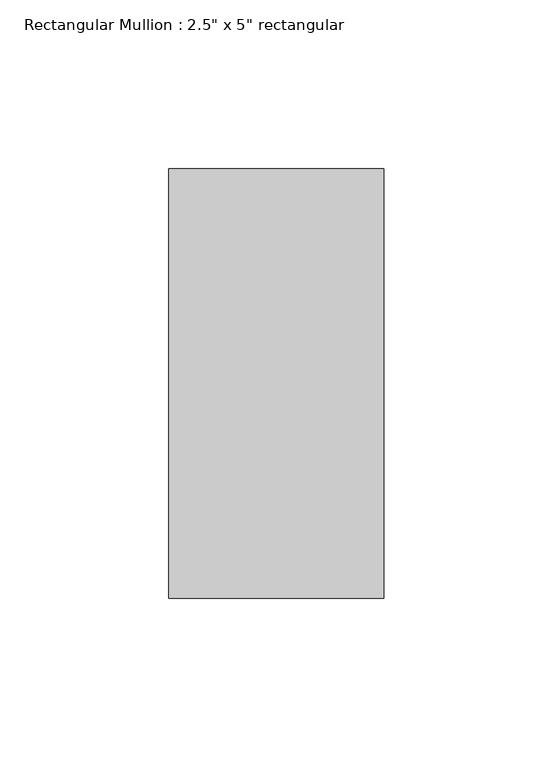
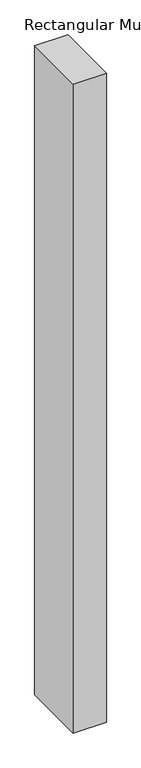
"""IFC4 building model written with IfcOpenShell, lengths in millimetres: member geometry."""

from ifc_helpers import new_model, si_unit, frame, origin, place, context, project, spatial, polyline, outline, extrude, source, transform, mapped, element, save


def member_f9f7e124(model_context):
    return source(origin(), model_context, "Body", "SweptSolid", [
        extrude(outline(polyline([(31.75, 63.5), (31.75, -63.5), (-31.75, -63.5), (-31.75, 63.5), (31.75, 63.5)])), frame((0.0, 0.0, -1310.2166668), z_axis=(0.0, 0.0, 1.0), x_axis=(1.0, 0.0, 0.0)), (0.0, 0.0, 1.0), 1310.2166668),
    ])


if __name__ == "__main__":
    model = new_model("IFC4")
    model_context = context("Model", 3, world=origin())
    ifc_project = project(units=[si_unit("LENGTHUNIT", "METRE", prefix="MILLI")], contexts=[model_context])
    site = spatial("IfcSite", under=ifc_project)
    building = spatial("IfcBuilding", under=site)
    placement = place(None, origin())
    member_shape = member_f9f7e124(model_context)
    element("IfcMember", 1, ObjectType="Rectangular Mullion : 2.5\" x 5\" rectangular", at=placement, inside=building, context=model_context, shape_type="MappedRepresentation", body=[
        mapped(member_shape, transform((0.0, 0.0, 0.0), x_axis=(1.0, 0.0, 0.0), y_axis=(0.0, 1.0, 0.0), z_axis=(0.0, 0.0, 1.0))),
    ])
    save(model, "model.ifc")

# Revit data of these elements
# Type "Rectangular Mullion : 2.5\" x 5\" rectangular"
#   built-in parameter 1007304 = 0.416667 (stored number, unit not read)
#   built-in parameter 1007301 = 0.104167 (stored number, unit not read)
#   built-in parameter 1007300 = 0.104167 (stored number, unit not read)
# Element 1 (IfcMember, "Rectangular Mullion : 2.5\" x 5\" rectangular")
#   Materials on its faces: "Aluminum"
# Materials
#   "Aluminum": class "Metal", colour RGB 247 247 247, transparency 0, Description = "Aluminum 6061", Cost = 0
